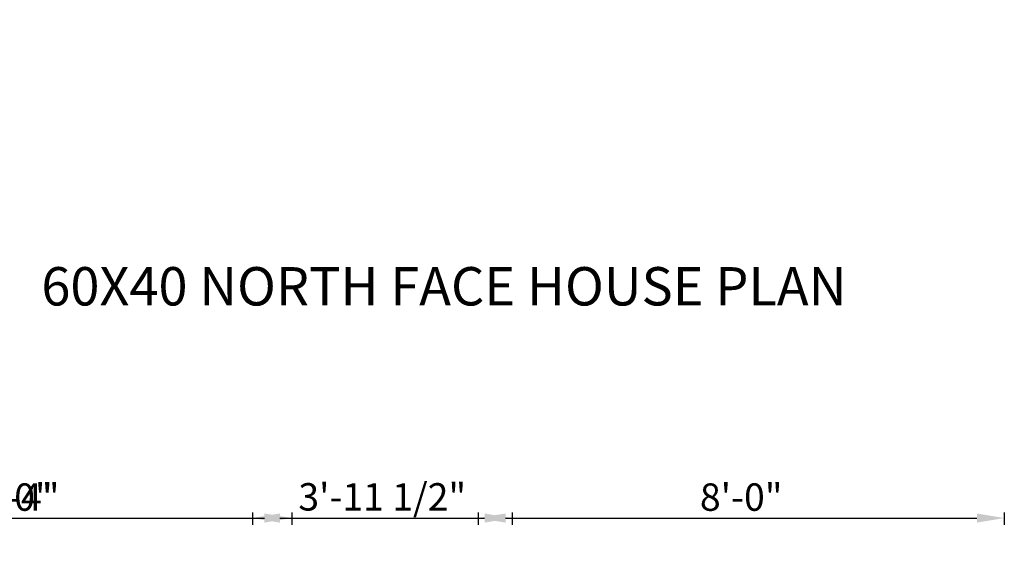
# Model space of a CAD drawing. Units: inches. Extents: x -100 to 766, y -562 to 63.
# Tile 3 of 11: x 268 to 448, y -562 to -467. Entities that reach past the tile are written whole.
import ezdxf

# ---------------------------------------------------------------- set-up
doc = ezdxf.new("R2010")
doc.units = ezdxf.units.IN
doc.layers.add('A-ANNO-DIMS', color=2, linetype='Continuous', lineweight=18)
doc.layers.add('A-ANNO-TEXT', color=7, linetype='Continuous', lineweight=18)
doc.styles.get("Standard").update_dxf_attribs({"font": 'arial.ttf'})
doc.dimstyles.new('ISO-25', dxfattribs={"dimtxt": 5, "dimasz": 5, "dimexe": 1.25, "dimexo": 0.625, "dimtad": 1, "dimlunit": 3, "dimtxsty": 'Standard', "dimcen": 2.5, "dimadec": 0, "dimazin": 0, "dimtfac": 1, "dimtmove": 0, "dimatfit": 3, "dimfxl": 1, "dimfxlon": 1, "dimarcsym": 0})

# ---------------------------------------------------------------- blocks, each defined once
blk = doc.blocks.new('*D22')
at = {"layer": 'A-ANNO-DIMS', "color": 0, "lineweight": -2, "transparency": 16777216}
for p, q in [((193.47, -456.51), (193.47, -454.26)), ((211.47, -456.51), (211.47, -454.26)), ((198.47, -455.51), (206.47, -455.51)), ((211.47, -455.51), (287.98, -455.51))]:
    blk.add_line(p, q, dxfattribs=at)
at = {"layer": 'A-ANNO-DIMS', "color": 0, "transparency": 16777216}
for points in [[(198.47, -454.68), (198.47, -456.35), (193.47, -455.51)], [(206.47, -454.68), (206.47, -456.35), (211.47, -455.51)]]:
    blk.add_solid(points, dxfattribs=at)
at = {"layer": 'Defpoints', "color": 0, "transparency": 16777216}
for p in [(211.47, -455.51), (193.47, -458.21), (211.47, -458.21)]:
    blk.add_point(p, dxfattribs=at)
at = {"layer": 'A-ANNO-DIMS', "color": 0, "transparency": 16777216, "insert": (252.23, -452.3), "char_height": 5, "attachment_point": 5}
blk.add_mtext('WINDOW C 1\'-6" TYP.', dxfattribs=at)
blk = doc.blocks.new('*D67')
at = {"layer": 'A-ANNO-DIMS', "color": 0, "lineweight": -2, "transparency": 16777216}
for p, q in [((211.47, -557.16), (211.47, -559.41)), ((216.47, -558.16), (312.6, -558.16)), ((317.6, -557.16), (317.6, -559.41))]:
    blk.add_line(p, q, dxfattribs=at)
at = {"layer": 'A-ANNO-DIMS', "color": 0, "transparency": 16777216}
for points in [[(216.47, -557.32), (216.47, -558.99), (211.47, -558.16)], [(312.6, -557.32), (312.6, -558.99), (317.6, -558.16)]]:
    blk.add_solid(points, dxfattribs=at)
at = {"layer": 'Defpoints', "color": 0, "transparency": 16777216}
for p in [(211.47, -467.21), (317.6, -467.21), (317.6, -558.16)]:
    blk.add_point(p, dxfattribs=at)
at = {"layer": 'A-ANNO-DIMS', "color": 0, "transparency": 16777216, "insert": (264.53, -554.98), "char_height": 5, "attachment_point": 5}
blk.add_mtext('8\'-10"', dxfattribs=at)
blk = doc.blocks.new('*D68')
at = {"layer": 'A-ANNO-DIMS', "color": 0, "lineweight": -2, "transparency": 16777216}
for p, q in [((351.6, -557.16), (351.6, -559.41)), ((356.6, -558.16), (442.62, -558.16)), ((447.62, -557.16), (447.62, -559.41))]:
    blk.add_line(p, q, dxfattribs=at)
at = {"layer": 'A-ANNO-DIMS', "color": 0, "transparency": 16777216}
for points in [[(356.6, -557.32), (356.6, -558.99), (351.6, -558.16)], [(442.62, -557.32), (442.62, -558.99), (447.62, -558.16)]]:
    blk.add_solid(points, dxfattribs=at)
at = {"layer": 'Defpoints', "color": 0, "transparency": 16777216}
for p in [(351.6, -467.21), (447.62, -467.29), (447.62, -558.16)]:
    blk.add_point(p, dxfattribs=at)
at = {"layer": 'A-ANNO-DIMS', "color": 0, "transparency": 16777216, "insert": (399.61, -554.98), "char_height": 5, "attachment_point": 5}
blk.add_mtext('8\'-0"', dxfattribs=at)
blk = doc.blocks.new('*D80')
at = {"layer": 'A-ANNO-DIMS', "color": 0, "lineweight": -2, "transparency": 16777216}
for p, q in [((241.52, -558.16), (236.52, -558.16)), ((246.52, -557.16), (246.52, -559.41)), ((246.52, -558.16), (250.39, -558.16)), ((250.39, -557.16), (250.39, -559.41)), ((255.39, -558.16), (274.93, -558.16))]:
    blk.add_line(p, q, dxfattribs=at)
at = {"layer": 'A-ANNO-DIMS', "color": 0, "transparency": 16777216}
for points in [[(241.52, -557.32), (241.52, -558.99), (246.52, -558.16)], [(255.39, -557.32), (255.39, -558.99), (250.39, -558.16)]]:
    blk.add_solid(points, dxfattribs=at)
at = {"layer": 'Defpoints', "color": 0, "transparency": 16777216}
for p in [(246.52, -368.21), (250.39, -368.21), (250.39, -558.16)]:
    blk.add_point(p, dxfattribs=at)
at = {"layer": 'A-ANNO-DIMS', "color": 0, "transparency": 16777216, "insert": (267.66, -554.98), "char_height": 5, "attachment_point": 5}
blk.add_mtext('0\'-4"', dxfattribs=at)
blk = doc.blocks.new('*D87')
at = {"layer": 'A-ANNO-DIMS', "color": 0, "lineweight": -2, "transparency": 16777216}
for p, q in [((310.41, -557.16), (310.41, -559.41)), ((315.41, -558.16), (352.79, -558.16)), ((357.79, -557.16), (357.79, -559.41))]:
    blk.add_line(p, q, dxfattribs=at)
at = {"layer": 'A-ANNO-DIMS', "color": 0, "transparency": 16777216}
for points in [[(315.41, -557.32), (315.41, -558.99), (310.41, -558.16)], [(352.79, -557.32), (352.79, -558.99), (357.79, -558.16)]]:
    blk.add_solid(points, dxfattribs=at)
at = {"layer": 'Defpoints', "color": 0, "transparency": 16777216}
for p in [(310.41, -121.91), (357.79, -121.91), (357.79, -558.16)]:
    blk.add_point(p, dxfattribs=at)
at = {"layer": 'A-ANNO-DIMS', "color": 0, "transparency": 16777216, "insert": (334.1, -554.94), "char_height": 5, "attachment_point": 5}
blk.add_mtext('3\'-11 1/2"', dxfattribs=at)

msp = doc.modelspace()

# ---------------------------------------------------------------- texts
at = {"layer": 'A-ANNO-TEXT', "insert": (271.89, -512.364), "char_height": 7, "attachment_point": 1}
msp.add_mtext_dynamic_manual_height_columns('60X40 NORTH FACE HOUSE PLAN', width=552.24461, gutter_width=12.5, heights=[0], dxfattribs=at)

# ---------------------------------------------------------------- dimensions: what is measured, and where the dimension line sits
at = {"layer": 'A-ANNO-DIMS'}
for base, p1, p2, picture, middle in [((357.792, -558.156), (310.414, -121.911), (357.792, -121.911), '*D87', (334.103, -554.944)), ((250.388, -558.156), (246.522, -368.214), (250.388, -368.214), '*D80', (267.658, -554.979)), ((317.595, -558.156), (211.473, -467.214), (317.595, -467.214), '*D67', (264.534, -554.979)), ((447.624, -558.156), (351.595, -467.214), (447.624, -467.288), '*D68', (399.609, -554.979))]:
    dim = msp.add_linear_dim(base=base, p1=p1, p2=p2, dimstyle='ISO-25', override={"dimdec": 1, "dimlfac": 1, "dimrnd": 0, "dimzin": 1, "dimdsep": 46, "dimlunit": 4, "dimfrac": 2}, dxfattribs=at)
    dim.commit()
    dim.dimension.update_dxf_attribs({"geometry": picture, "text_midpoint": middle})
dim = msp.add_linear_dim(base=(211.473, -455.514), p1=(193.473, -458.214), p2=(211.473, -458.214), angle=0, text='WINDOW C <> TYP.', dimstyle='ISO-25', override={"dimdec": 1, "dimlfac": 1, "dimrnd": 0, "dimzin": 1, "dimdsep": 46, "dimlunit": 4, "dimfrac": 2}, dxfattribs=at)
dim.commit()
dim.dimension.update_dxf_attribs({"geometry": '*D22', "text_midpoint": (252.226, -452.302)})

doc.saveas('drawing.dxf')
